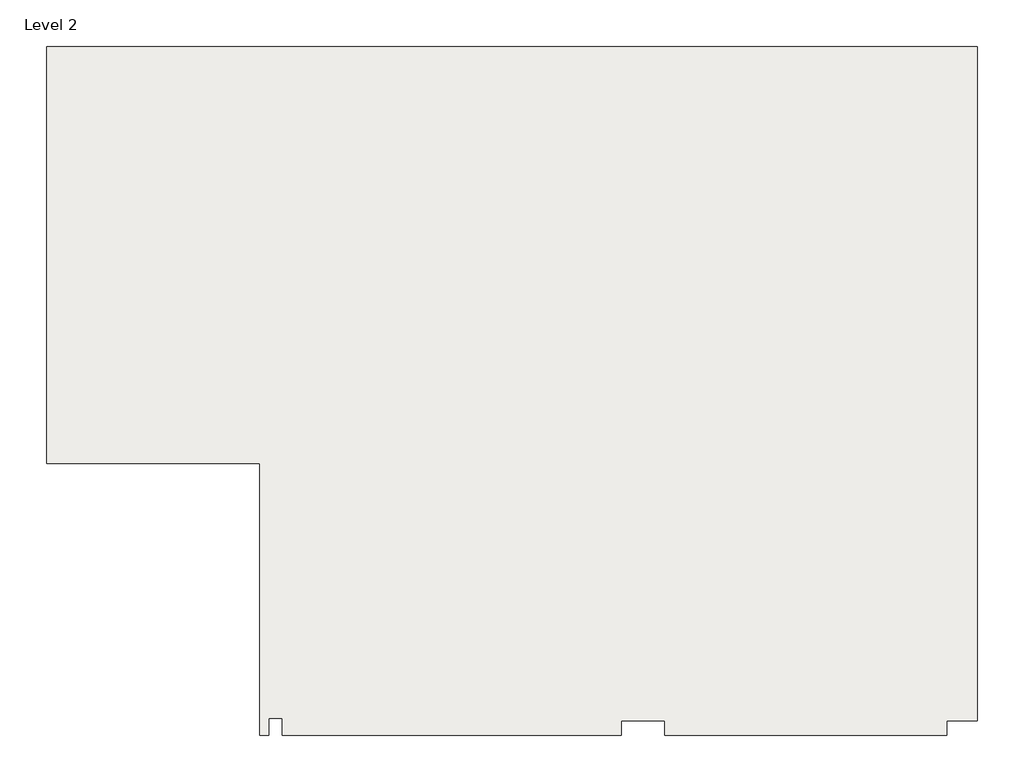
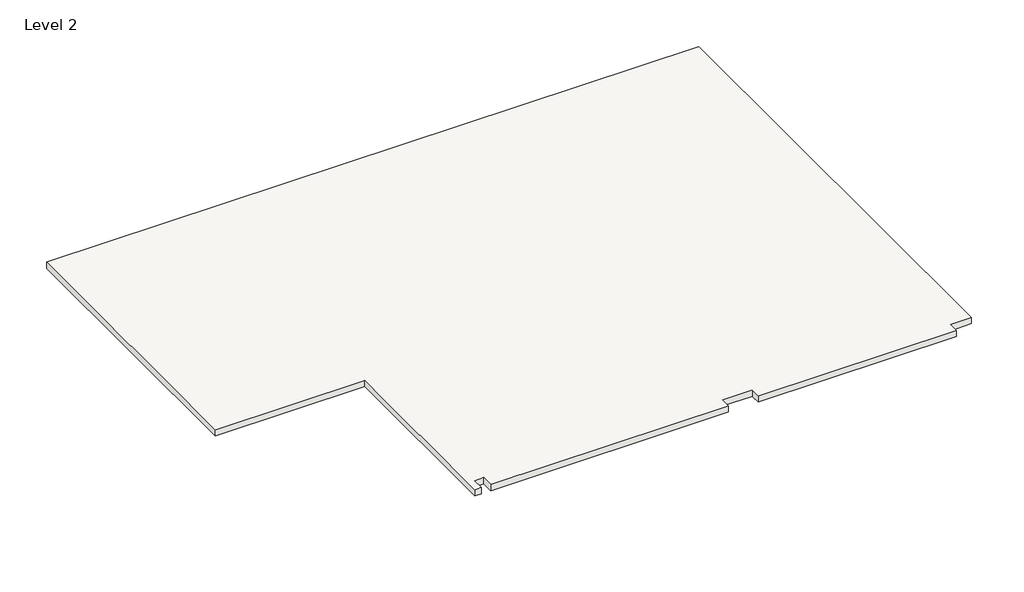
# One storey: 1 roof.
"""IFC4 building model written with IfcOpenShell, lengths in millimetres."""

from ifc_helpers import new_model, si_unit, frame, origin, place, context, project, spatial, polyline, outline, extrude, element, save

model = new_model("IFC4")

# Units and contexts
model_context = context("Model", 3, world=origin())
ifc_project = project(units=[si_unit("LENGTHUNIT", "METRE", prefix="MILLI")], contexts=[model_context])

# Site, building, storey
site = spatial("IfcSite", under=ifc_project)
building = spatial("IfcBuilding", under=site)
storey = spatial("IfcBuildingStorey", under=building, Name="Level 2", Elevation=3048.0)

# Roof
placement = place(None, origin())
element("IfcRoof", 1, ObjectType="Wood Rafter 8\" - Asphalt Shingle - Insulated", at=placement, inside=storey, context=model_context, shape_type="SweptSolid", body=[
    extrude(outline(polyline([(-20180.4480019, 5318.0258877), (-20180.4480019, 14665.2258877), (672.9519981, 14665.2258877), (672.9519981, -447.7741123), (-12.8480019, -447.7741123), (-12.8480019, -777.9741123), (-6337.4480019, -777.9741123), (-6337.4480019, -447.7741123), (-7302.6480019, -447.7741123), (-7302.6480019, -777.9741123), (-14897.2480019, -777.9741123), (-14897.2480019, -396.9741123), (-15202.0480019, -396.9741123), (-15202.0480019, -777.9741123), (-15405.2480019, -777.9741123), (-15405.2480019, 5318.0258877), (-20180.4480019, 5318.0258877)])), frame((0.0, 0.0, 3048.0), z_axis=(0.0, 0.0, 1.0), x_axis=(1.0, 0.0, 0.0)), (0.0, 0.0, 1.0), 212.725),
])

save(model, "model.ifc")

# Revit data of these elements
# Type "Wood Rafter 8\" - Asphalt Shingle - Insulated"
#   Assembly Code = "B1020"
#   Layers, outside or top first: 0' - 0 1/4" "Asphalt Shingle" (function 4); 0' - 0 5/8" "Plywood, Sheathing" (function 2); 0' - 7 1/2" "Structure, Wood Joist/Rafter Layer, Batt Insulation" (function 1)
# Element 1 (IfcRoof, "Wood Rafter 8\" - Asphalt Shingle - Insulated")
#   built-in parameter 1001705 = 10.6979 (stored number, unit not read)
#   built-in parameter 1001710 = 33615
#   Phase Created = New Construction
#   Materials on its faces: "Structure, Wood Joist/Rafter Layer, Batt Insulation", "Asphalt Shingle"
# Materials
#   "Asphalt Shingle": class "Generic", colour RGB 155 155 155, transparency 0, Description = "Asphalt roofing shingle", Cost = 0
#   "Plywood, Sheathing": class "Wood", colour RGB 212 179 113, transparency 0, Description = "Plywood, sheathing grade", Cost = 0
#   "Structure, Wood Joist/Rafter Layer, Batt Insulation": class "Wood", colour RGB 127 127 127, transparency 0, Description = "Wood framing, insulated", Cost = 0
